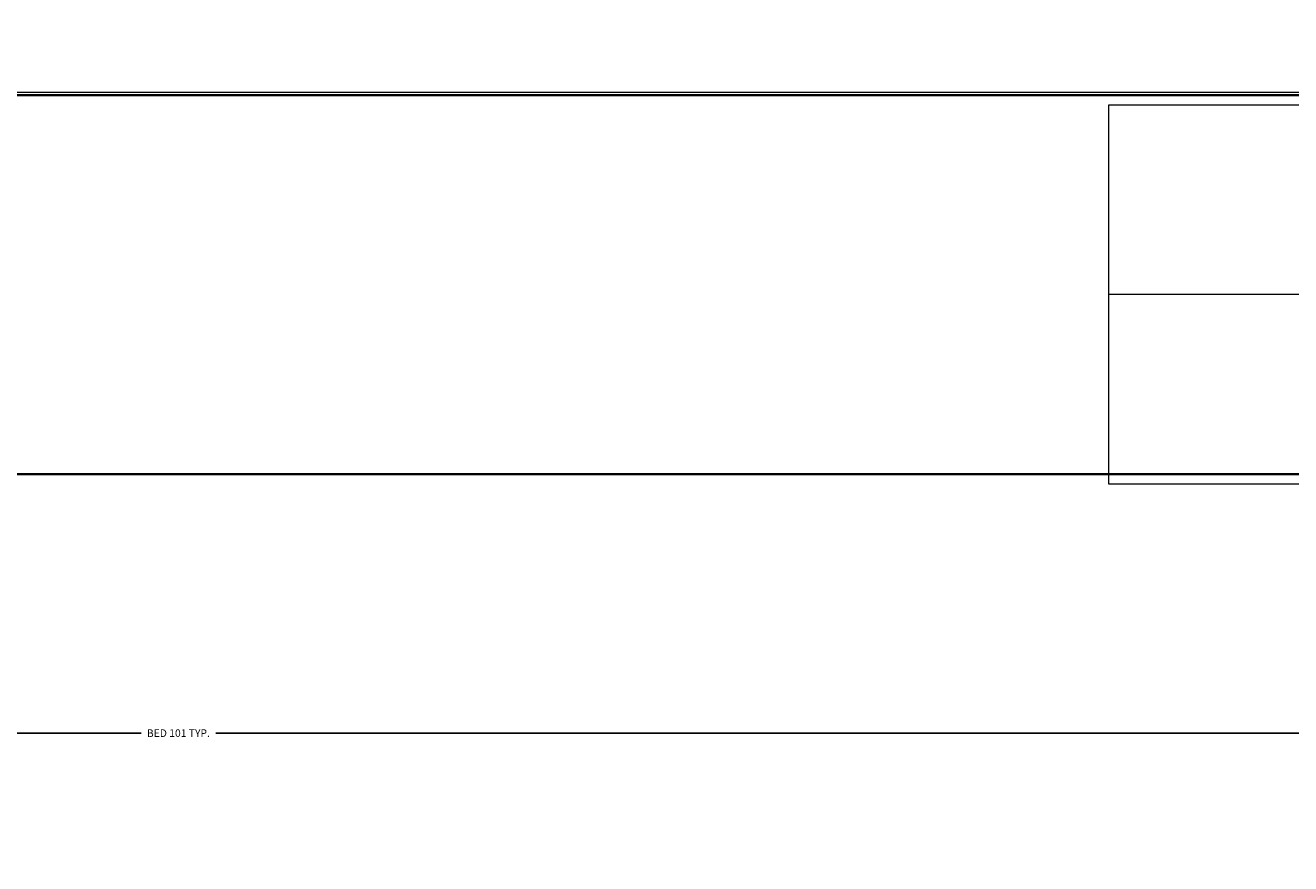
# Model space of a CAD drawing. Units: millimetres. Extents: x 27017497 to 27018854, y 7058029 to 7059154.
# Tile 23 of 91: x 27017702 to 27017732, y 7058124 to 7058144. Entities that reach past the tile are written whole.
import ezdxf

# ---------------------------------------------------------------- set-up
doc = ezdxf.new("R2010")
doc.units = ezdxf.units.MM
for name, color, linetype, lineweight in [('A-ANNO-DIMS', 2, 'Continuous', 18), ('A-FURN', 8, 'Continuous', 18), ('A-GLAZ', 4, 'Continuous', 18), ('A-WALL', 7, 'Continuous', 35)]:
    doc.layers.add(name, color=color, linetype=linetype, lineweight=lineweight)
doc.styles.get("Standard").update_dxf_attribs({"font": 'arial.ttf'})
doc.dimstyles.get("Standard").update_dxf_attribs({"dimtxt": 0.18, "dimasz": 0.18, "dimexe": 0.18, "dimexo": 0.0625, "dimgap": 0.09, "dimtad": 0, "dimtih": 1, "dimtoh": 1, "dimdec": 4, "dimzin": 0, "dimdsep": 46, "dimtxsty": 'Standard', "dimcen": 0.09, "dimadec": 0, "dimazin": 0, "dimtfac": 1, "dimtdec": 4, "dimtofl": 0, "dimtmove": 0, "dimatfit": 3, "dimfxl": 1, "dimtolj": 1, "dimtzin": 0, "dimarcsym": 0})

# ---------------------------------------------------------------- blocks, each defined once
blk = doc.blocks.new('CAMMAT')
blk.add_line((1.27313, 0), (-1.27313, 0))
blk = doc.blocks.new('WINDOW-SINGLE-LIGHT')
blk.add_lwpolyline([(36, 4.5), (36, 0), (0, 0), (0, 9), (36, 9), (36, 4.5), (0, 4.5)])
blk = doc.blocks.new('*D25')
at = {"layer": 'A-ANNO-DIMS', "color": 0, "lineweight": -2, "transparency": 16777216}
for p, q in [((27017654.932, 7058141.917), (27017654.932, 7058126.587)), ((27017756.349, 7058141.917), (27017756.349, 7058126.587)), ((27017655.112, 7058126.767), (27017704.753, 7058126.767)), ((27017756.169, 7058126.767), (27017706.528, 7058126.767))]:
    blk.add_line(p, q, dxfattribs=at)
at = {"layer": 'A-ANNO-DIMS', "color": 0, "transparency": 16777216}
for points in [[(27017655.112, 7058126.797), (27017655.112, 7058126.737), (27017654.932, 7058126.767)], [(27017756.169, 7058126.797), (27017756.169, 7058126.737), (27017756.349, 7058126.767)]]:
    blk.add_solid(points, dxfattribs=at)
at = {"layer": 'Defpoints', "color": 0, "transparency": 16777216}
for p in [(27017654.932, 7058141.98), (27017756.349, 7058141.98), (27017654.932, 7058126.767)]:
    blk.add_point(p, dxfattribs=at)
at = {"layer": 'A-ANNO-DIMS', "color": 0, "transparency": 16777216, "insert": (27017705.64, 7058126.767), "char_height": 0.18, "attachment_point": 5}
blk.add_mtext('\\A1;BED 101 TYP.', dxfattribs=at)
blk = doc.blocks.new('*D47')
at = {"layer": 'A-ANNO-DIMS', "color": 0, "lineweight": -2, "transparency": 16777216}
for p, q in [((27017561.166, 7058294.35), (27017561.166, 7058028.6)), ((27018790.606, 7058294.35), (27018790.606, 7058028.6)), ((27017561.346, 7058028.78), (27018175.431, 7058028.78)), ((27018790.426, 7058028.78), (27018176.341, 7058028.78))]:
    blk.add_line(p, q, dxfattribs=at)
at = {"layer": 'A-ANNO-DIMS', "color": 0, "transparency": 16777216}
for points in [[(27017561.346, 7058028.81), (27017561.346, 7058028.75), (27017561.166, 7058028.78)], [(27018790.426, 7058028.81), (27018790.426, 7058028.75), (27018790.606, 7058028.78)]]:
    blk.add_solid(points, dxfattribs=at)
at = {"layer": 'Defpoints', "color": 0, "transparency": 16777216}
for p in [(27017561.166, 7058294.412), (27018790.606, 7058294.412), (27018790.606, 7058028.78)]:
    blk.add_point(p, dxfattribs=at)
at = {"layer": 'A-ANNO-DIMS', "color": 0, "transparency": 16777216, "insert": (27018175.886, 7058028.78), "char_height": 0.18, "attachment_point": 5}
blk.add_mtext('\\A1;1229.4', dxfattribs=at)
blk = doc.blocks.new('*D48')
at = {"layer": 'A-ANNO-DIMS', "color": 0, "lineweight": -2, "transparency": 16777216}
for p, q in [((27018463.498, 7058622.912), (27017497.536, 7058622.912)), ((27017497.716, 7058622.732), (27017497.716, 7058357.753)), ((27017497.716, 7058092.41), (27017497.716, 7058357.389)), ((27018555.129, 7058092.23), (27017497.536, 7058092.23))]:
    blk.add_line(p, q, dxfattribs=at)
at = {"layer": 'A-ANNO-DIMS', "color": 0, "transparency": 16777216}
for points in [[(27017497.686, 7058622.732), (27017497.746, 7058622.732), (27017497.716, 7058622.912)], [(27017497.686, 7058092.41), (27017497.746, 7058092.41), (27017497.716, 7058092.23)]]:
    blk.add_solid(points, dxfattribs=at)
at = {"layer": 'Defpoints', "color": 0, "transparency": 16777216}
for p in [(27018463.561, 7058622.912), (27017497.716, 7058092.23), (27018555.192, 7058092.23)]:
    blk.add_point(p, dxfattribs=at)
at = {"layer": 'A-ANNO-DIMS', "color": 0, "transparency": 16777216, "insert": (27017497.716, 7058357.571), "char_height": 0.18, "attachment_point": 5}
blk.add_mtext('\\A1;530.7', dxfattribs=at)

msp = doc.modelspace()

# ---------------------------------------------------------------- linework, layer by layer
at = {"layer": 'A-WALL'}
for p, q in [((27017622.666, 7058141.912), (27017802.166, 7058141.912)), ((27017613.666, 7058132.912), (27017802.166, 7058132.912)), ((27017613.666, 7058132.912), (27017802.166, 7058132.912))]:
    msp.add_line(p, q, dxfattribs=at)

# ---------------------------------------------------------------- block references
at = {"layer": 'A-FURN', "xscale": 39.82996475819422, "yscale": 39.82996475819422, "zscale": 39.82996475819422, "rotation": 180}
msp.add_blockref('CAMMAT', (27017705.64, 7058141.98), dxfattribs=at)
at = {"layer": 'A-GLAZ'}
msp.add_blockref('WINDOW-SINGLE-LIGHT', (27017727.724, 7058132.679), dxfattribs=at)

# ---------------------------------------------------------------- dimensions: what is measured, and where the dimension line sits
at = {"layer": 'A-ANNO-DIMS'}
dim = msp.add_linear_dim(base=(27017497.716, 7058092.23), p1=(27018463.561, 7058622.912), p2=(27018555.192, 7058092.23), angle=90, dimstyle='Standard', override={"dimdec": 1, "dimlfac": 1, "dimrnd": 0, "dimzin": 0, "dimdsep": 46, "dimlunit": 2}, dxfattribs=at)
dim.commit()
dim.dimension.update_dxf_attribs({"geometry": '*D48', "text_midpoint": (27017497.716, 7058357.571)})
dim = msp.add_linear_dim(base=(27018790.606, 7058028.78), p1=(27017561.166, 7058294.412), p2=(27018790.606, 7058294.412), dimstyle='Standard', override={"dimdec": 1, "dimlfac": 1, "dimrnd": 0, "dimzin": 0, "dimdsep": 46, "dimlunit": 2}, dxfattribs=at)
dim.commit()
dim.dimension.update_dxf_attribs({"geometry": '*D47', "text_midpoint": (27018175.886, 7058028.78)})
dim = msp.add_linear_dim(base=(27017654.932, 7058126.767), p1=(27017756.349, 7058141.98), p2=(27017654.932, 7058141.98), angle=180, text='BED <> TYP.', dimstyle='Standard', override={"dimdec": 0, "dimlfac": 1, "dimrnd": 0, "dimzin": 0, "dimdsep": 46, "dimlunit": 2}, dxfattribs=at)
dim.commit()
dim.dimension.update_dxf_attribs({"geometry": '*D25', "text_midpoint": (27017705.64, 7058126.767)})

doc.saveas('drawing.dxf')
